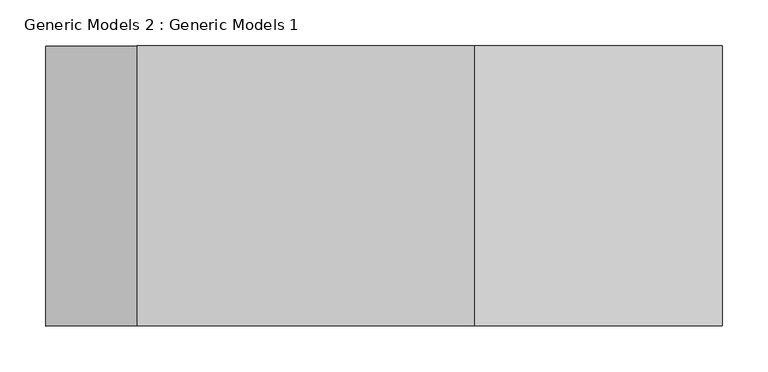
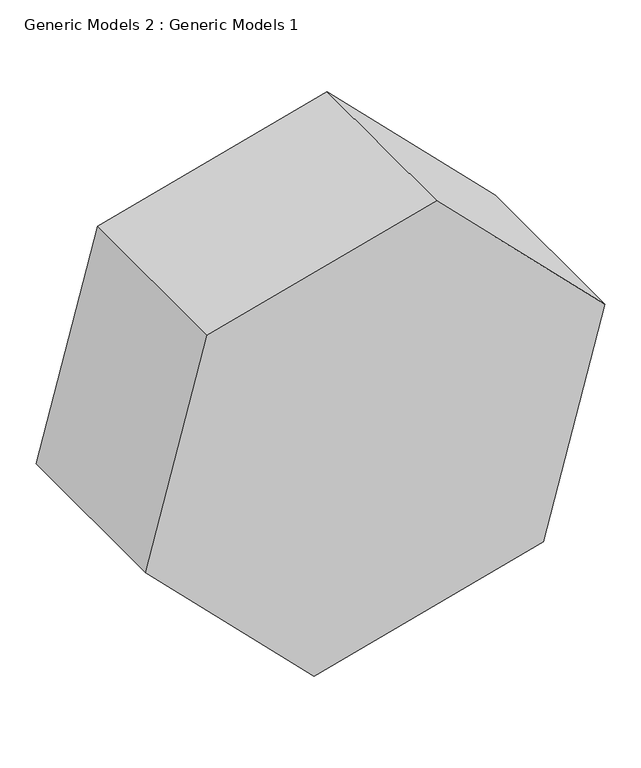
"""IFC4 building model written with IfcOpenShell, lengths in millimetres: proxy geometry, Generic Models 2 : Generic Models 1."""

from ifc_helpers import new_model, si_unit, frame, origin, place, context, project, spatial, polyline, outline, extrude, source, transform, mapped, element, save


def generic_models_2_generic_models_1_f357a12c(model_context):
    return source(origin(), model_context, "Body", "SweptSolid", [
        extrude(outline(polyline([(708.0393724, -5688.8273199), (977.447056, -5958.2350036), (878.8369998, -6326.2527434), (510.81926, -6424.8627996), (241.4115764, -6155.4551159), (340.0216325, -5787.4373761), (708.0393724, -5688.8273199)])), frame((0.0, -10102.5989753, 0.0), z_axis=(0.0, 1.0, 0.0), x_axis=(0.0, 0.0, 1.0)), (0.0, 0.0, 1.0), 304.8),
    ])


if __name__ == "__main__":
    model = new_model("IFC4")
    model_context = context("Model", 3, world=origin())
    ifc_project = project(units=[si_unit("LENGTHUNIT", "METRE", prefix="MILLI")], contexts=[model_context])
    site = spatial("IfcSite", under=ifc_project)
    building = spatial("IfcBuilding", under=site)
    placement = place(None, origin())
    generic_models_2_generic_models_1_shape = generic_models_2_generic_models_1_f357a12c(model_context)
    element("IfcBuildingElementProxy", 1, Name="Generic Models 2 : Generic Models 1", ObjectType="Generic Models 2 : Generic Models 1", at=placement, inside=building, context=model_context, shape_type="MappedRepresentation", body=[
        mapped(generic_models_2_generic_models_1_shape, transform((0.0, 0.0, 0.0), x_axis=(1.0, 0.0, 0.0), y_axis=(0.0, 1.0, 0.0), z_axis=(0.0, 0.0, 1.0))),
    ])
    save(model, "model.ifc")

# Revit data of these elements
# Element 1 (IfcBuildingElementProxy, "Generic Models 2 : Generic Models 1")
#   Materials on its faces: "Carpet (1)"
# Materials
#   "Carpet (1)": class "Carpet", colour RGB 124 80 67, transparency 0, Description = "Interior finish", Cost = 0
